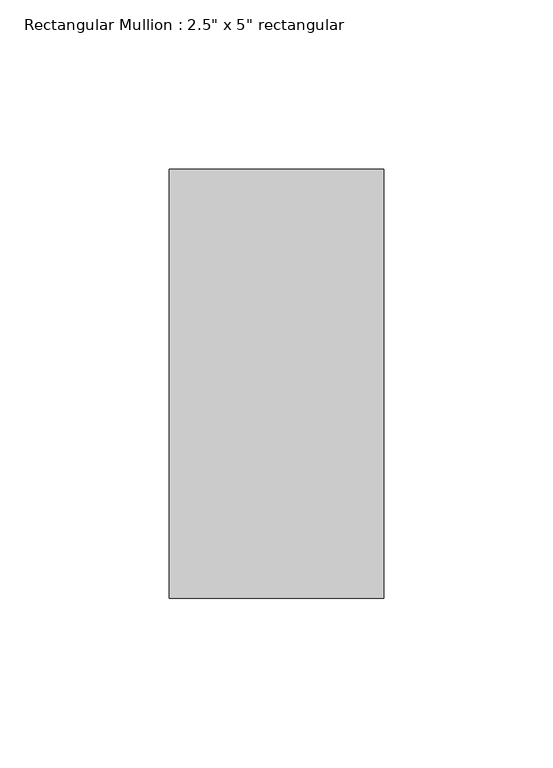
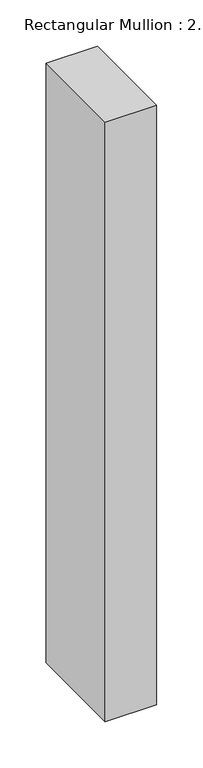
"""IFC4 building model written with IfcOpenShell, lengths in millimetres: member geometry."""

from ifc_helpers import new_model, si_unit, frame, origin, place, context, project, spatial, polyline, outline, extrude, source, transform, mapped, element, save


def member_429f6687(model_context):
    return source(origin(), model_context, "Body", "SweptSolid", [
        extrude(outline(polyline([(0.0, 63.5), (0.0, -63.5), (-63.5, -63.5), (-63.5, 63.5), (0.0, 63.5)])), frame((0.0, 0.0, -787.4), z_axis=(0.0, 0.0, 1.0), x_axis=(1.0, 0.0, 0.0)), (0.0, 0.0, 1.0), 787.4),
    ])


if __name__ == "__main__":
    model = new_model("IFC4")
    model_context = context("Model", 3, world=origin())
    ifc_project = project(units=[si_unit("LENGTHUNIT", "METRE", prefix="MILLI")], contexts=[model_context])
    site = spatial("IfcSite", under=ifc_project)
    building = spatial("IfcBuilding", under=site)
    placement = place(None, origin())
    member_shape = member_429f6687(model_context)
    element("IfcMember", 1, ObjectType="Rectangular Mullion : 2.5\" x 5\" rectangular", at=placement, inside=building, context=model_context, shape_type="MappedRepresentation", body=[
        mapped(member_shape, transform((0.0, 0.0, 0.0), x_axis=(1.0, 0.0, 0.0), y_axis=(0.0, 1.0, 0.0), z_axis=(0.0, 0.0, 1.0))),
    ])
    save(model, "model.ifc")

# Revit data of these elements
# Type "Rectangular Mullion : 2.5\" x 5\" rectangular"
#   built-in parameter 1007304 = 0.416667 (stored number, unit not read)
#   built-in parameter 1007301 = 0.104167 (stored number, unit not read)
#   built-in parameter 1007300 = 0.104167 (stored number, unit not read)
